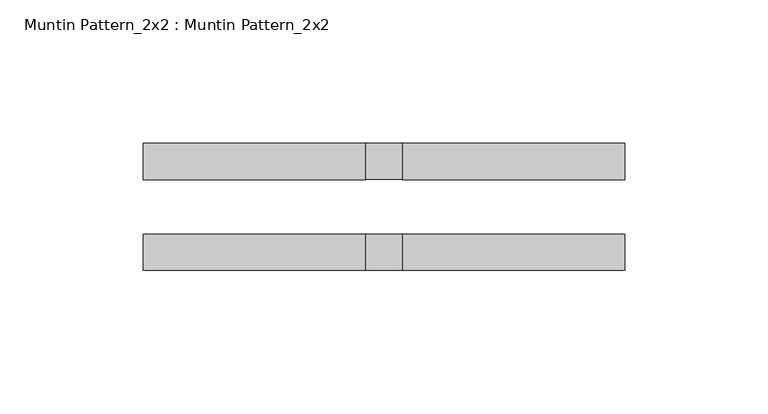
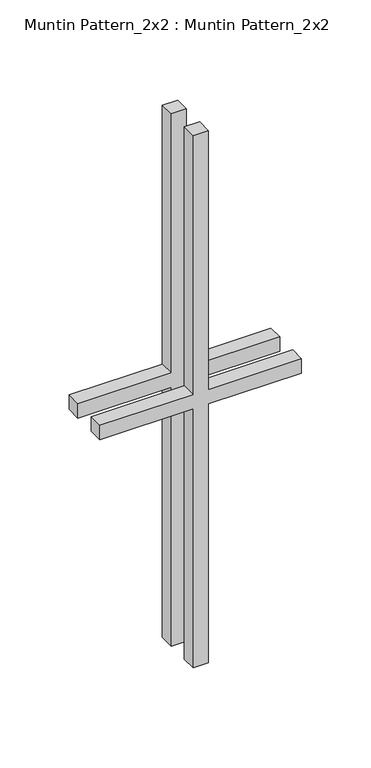
"""IFC4 building model written with IfcOpenShell, lengths in millimetres: proxy geometry, Muntin Pattern_2x2 : Muntin Pattern_2x2."""

from ifc_helpers import new_model, si_unit, frame, origin, place, context, project, spatial, polyline, outline, extrude, source, transform, mapped, element, save


def muntin_pattern_2x2_muntin_pattern_2x2_cae9449b(model_context):
    return source(origin(), model_context, "Body", "SweptSolid", [
        extrude(outline(polyline([(241.3, -6.35), (241.3, -84.1375), (228.6, -84.1375), (228.6, -6.35), (0.0, -6.35), (0.0, 6.35), (228.6, 6.35), (228.6, 84.1375), (241.3, 84.1375), (241.3, 6.35), (469.9, 6.35), (469.9, -6.35), (241.3, -6.35)])), frame((0.0, -22.225, 0.0), z_axis=(0.0, 1.0, 0.0), x_axis=(0.0, 0.0, 1.0)), (0.0, 0.0, 1.0), 12.7),
        extrude(outline(polyline([(241.3, -6.35), (241.3, -84.1375), (228.6, -84.1375), (228.6, -6.35), (0.0, -6.35), (0.0, 6.35), (228.6, 6.35), (228.6, 84.1375), (241.3, 84.1375), (241.3, 6.35), (469.9, 6.35), (469.9, -6.35), (241.3, -6.35)])), frame((0.0, 9.525, 0.0), z_axis=(0.0, 1.0, 0.0), x_axis=(0.0, 0.0, 1.0)), (0.0, 0.0, 1.0), 12.7),
    ])


if __name__ == "__main__":
    model = new_model("IFC4")
    model_context = context("Model", 3, world=origin())
    ifc_project = project(units=[si_unit("LENGTHUNIT", "METRE", prefix="MILLI")], contexts=[model_context])
    site = spatial("IfcSite", under=ifc_project)
    building = spatial("IfcBuilding", under=site)
    placement = place(None, origin())
    muntin_pattern_2x2_muntin_pattern_2x2_shape = muntin_pattern_2x2_muntin_pattern_2x2_cae9449b(model_context)
    element("IfcBuildingElementProxy", 1, Name="Muntin Pattern_2x2 : Muntin Pattern_2x2", ObjectType="Muntin Pattern_2x2 : Muntin Pattern_2x2", at=placement, inside=building, context=model_context, shape_type="MappedRepresentation", body=[
        mapped(muntin_pattern_2x2_muntin_pattern_2x2_shape, transform((0.0, 0.0, 0.0), x_axis=(1.0, 0.0, 0.0), y_axis=(0.0, 1.0, 0.0), z_axis=(0.0, 0.0, 1.0))),
    ])
    save(model, "model.ifc")

# Revit data of these elements
# Type "Muntin Pattern_2x2 : Muntin Pattern_2x2"
#   Width [instance default] = 4' - 0"
#   Thickness = 0' - 0 1/2"
#   Height [instance default] = 4' - 0"
#   Distance = 0' - 0 3/4"
#   Interior Material [instance default] = none
#   Exterior Material [instance default] = none
#   Default Elevation = 0
# Element 1 (IfcBuildingElementProxy, "Muntin Pattern_2x2 : Muntin Pattern_2x2")
#   Width = 0' - 6 5/8"
#   Height = 1' - 6 1/2"
#   Interior Material = Wood - Stained
#   Exterior Material = Clad - White
#   Materials on its faces: "Clad - White", "Wood - Stained"
# Materials
#   "Clad - White": class "Wood", colour RGB 242 242 238, transparency 0, Cost = 0
#   "Wood - Stained": class "Wood", colour RGB 224 178 126, transparency 0, Cost = 0
